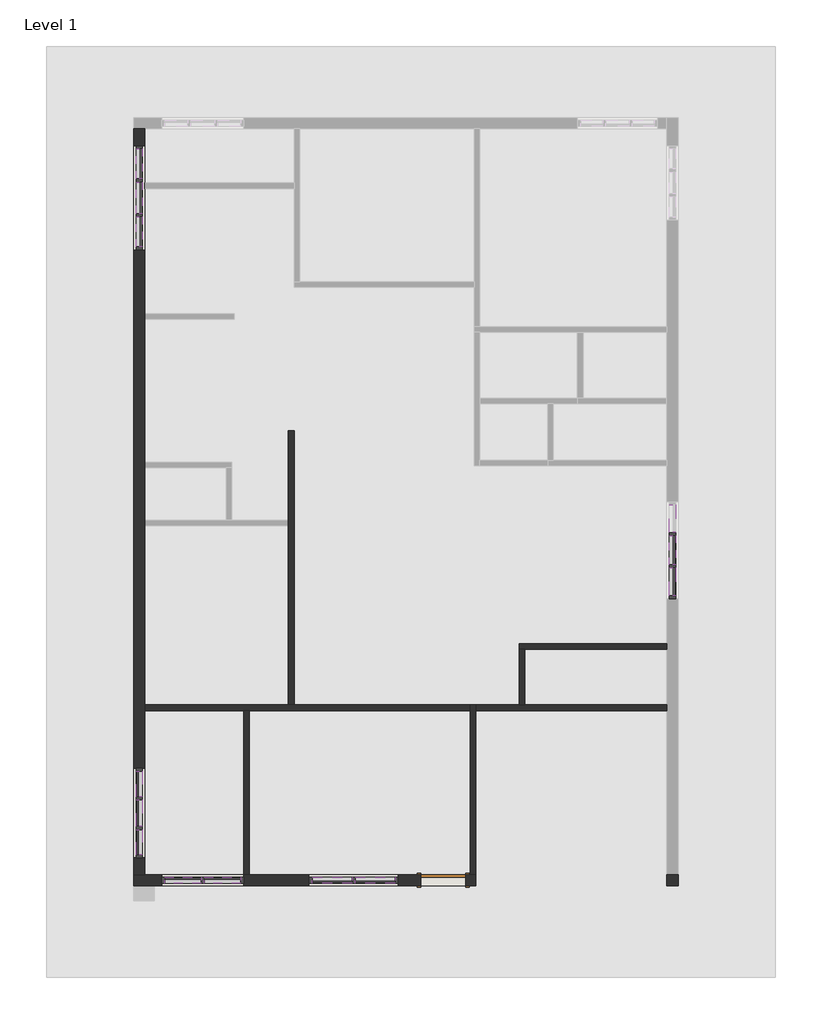
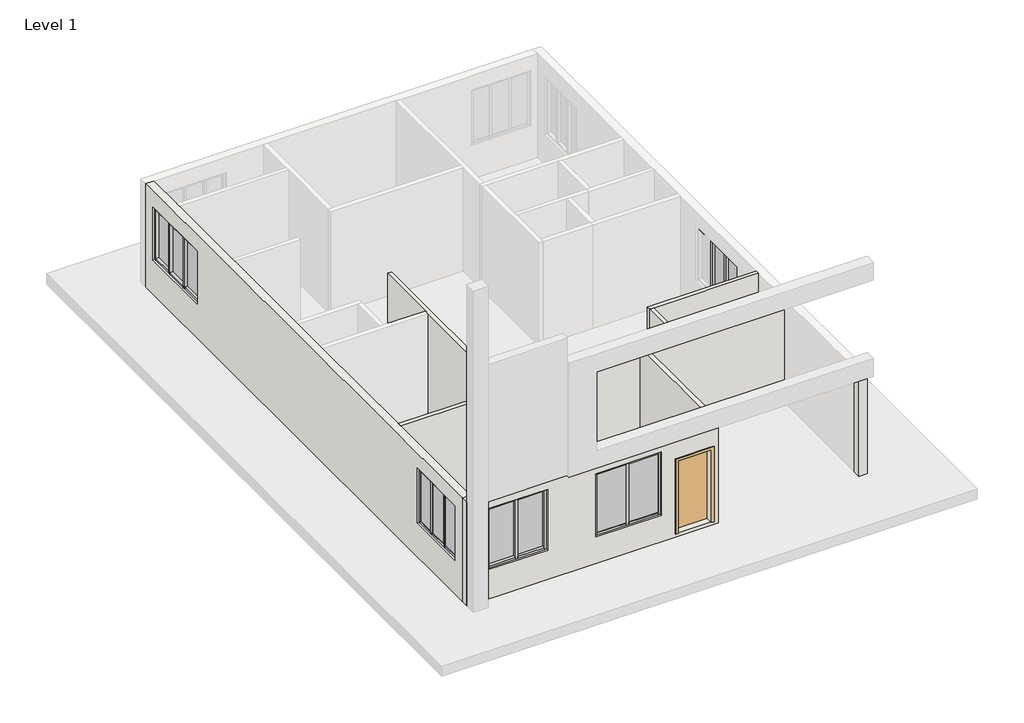
# One storey, part 1 of 2: 42 members, 12 plates, 10 walls, 1 door.
"""IFC4 building model written with IfcOpenShell, lengths in millimetres."""

from ifc_helpers import new_model, si_unit, origin, origin_with_axes, place, context, project, spatial, polyline, outline, extrude, faceted_brep, transform, mapped, element, save
from components import door_0ca8825f, member_6f432376, member_a400357f, member_9c3de6f4, member_520fb4b3, member_5215b92c, member_3f0e0172, member_3a7ae77e, member_6526e201, member_0b7646a3, member_196396ae, member_46a214c3, member_a980948f, member_c17f1be2, member_18118615, member_b3eff8b9, member_3a0a7659, member_3054d540, member_89344730, system_panel_glazed_22e8721b, system_panel_glazed_761c0abc, system_panel_glazed_28bcf516, system_panel_glazed_9d10e14a, system_panel_glazed_438a3505, system_panel_glazed_47776199, system_panel_glazed_6affd56b, system_panel_glazed_c6240b01

model = new_model("IFC4")

# Units and contexts
model_context = context("Model", 3, world=origin())
ifc_project = project(units=[si_unit("LENGTHUNIT", "METRE", prefix="MILLI")], contexts=[model_context])

# Site, building, storey
site = spatial("IfcSite", under=ifc_project)
building = spatial("IfcBuilding", under=site)
storey = spatial("IfcBuildingStorey", under=building, Name="Level 1", Elevation=0.0)

# Door
placement = place(None, origin())
door_shape = door_0ca8825f(model_context)
element("IfcDoor", 1, ObjectType="Single-Flush : 36\" x 84\"", at=placement, inside=storey, context=model_context, shape_type="MappedRepresentation", body=[
    mapped(door_shape, transform((-10676.5767684, -15219.4742702, 101.6), x_axis=(1.0, 0.0, 0.0), y_axis=(0.0, 1.0, 0.0), z_axis=(0.0, 0.0, 1.0))),
])

# Members
member_shape = member_6f432376(model_context)
element("IfcMember", 2, ObjectType="Rectangular Mullion : 2.5\" x 5\" rectangular", at=placement, inside=storey, context=model_context, shape_type="MappedRepresentation", body=[
    mapped(member_shape, transform((-5990.2767684, -8113.8242702, 2606.4568752), x_axis=(0.0, 0.0, 1.0), y_axis=(-1.0, 0.0, 0.0), z_axis=(0.0, -1.0, 0.0))),
])
element("IfcMember", 3, ObjectType="Rectangular Mullion : 2.5\" x 5\" rectangular", at=placement, inside=storey, context=model_context, shape_type="MappedRepresentation", body=[
    mapped(member_shape, transform((-5990.2767684, -9402.8742702, 2606.4568752), x_axis=(0.0, 0.0, 1.0), y_axis=(-1.0, 0.0, 0.0), z_axis=(0.0, -1.0, 0.0))),
])
member_2_shape = member_a400357f(model_context)
element("IfcMember", 4, ObjectType="Rectangular Mullion : 2.5\" x 5\" rectangular", at=placement, inside=storey, context=model_context, shape_type="MappedRepresentation", body=[
    mapped(member_2_shape, transform((-5990.2767684, -8774.2242702, 2606.4568752), x_axis=(0.0, 0.0, 1.0), y_axis=(-1.0, 0.0, 0.0), z_axis=(0.0, -1.0, 0.0))),
])
member_3_shape = member_9c3de6f4(model_context)
element("IfcMember", 5, ObjectType="Rectangular Mullion : 2.5\" x 5\" rectangular", at=placement, inside=storey, context=model_context, shape_type="MappedRepresentation", body=[
    mapped(member_3_shape, transform((-5990.2767684, -8145.5742702, 1004.9988244), x_axis=(0.0, -1.0, 0.0), y_axis=(-1.0, 0.0, 0.0), z_axis=(0.0, 0.0, -1.0))),
])
element("IfcMember", 6, ObjectType="Rectangular Mullion : 2.5\" x 5\" rectangular", at=placement, inside=storey, context=model_context, shape_type="MappedRepresentation", body=[
    mapped(member_3_shape, transform((-5990.2767684, -8805.9742702, 1004.9988244), x_axis=(0.0, -1.0, 0.0), y_axis=(-1.0, 0.0, 0.0), z_axis=(0.0, 0.0, -1.0))),
])
element("IfcMember", 7, ObjectType="Rectangular Mullion : 2.5\" x 5\" rectangular", at=placement, inside=storey, context=model_context, shape_type="MappedRepresentation", body=[
    mapped(member_2_shape, transform((-5990.2767684, -8177.3242702, 1004.9988244), x_axis=(0.0, 0.0, -1.0), y_axis=(-1.0, 0.0, 0.0), z_axis=(0.0, 1.0, 0.0))),
])
element("IfcMember", 8, ObjectType="Rectangular Mullion : 2.5\" x 5\" rectangular", at=placement, inside=storey, context=model_context, shape_type="MappedRepresentation", body=[
    mapped(member_shape, transform((-5990.2767684, -8837.7242702, 1004.9988244), x_axis=(0.0, 0.0, -1.0), y_axis=(-1.0, 0.0, 0.0), z_axis=(0.0, 1.0, 0.0))),
])
member_4_shape = member_520fb4b3(model_context)
element("IfcMember", 9, ObjectType="Rectangular Mullion : 2.5\" x 5\" rectangular", at=placement, inside=storey, context=model_context, shape_type="MappedRepresentation", body=[
    mapped(member_4_shape, transform((-5990.2767684, -9466.3742702, 1004.9988244), x_axis=(0.0, -1.0, 0.0), y_axis=(-1.0, 0.0, 0.0), z_axis=(0.0, 0.0, -1.0))),
])
member_5_shape = member_5215b92c(model_context)
element("IfcMember", 10, ObjectType="Rectangular Mullion : 2.5\" x 5\" rectangular", at=placement, inside=storey, context=model_context, shape_type="MappedRepresentation", body=[
    mapped(member_5_shape, transform((-16886.8767684, -1598.7242702, 2569.033555), x_axis=(0.0, 0.0, 1.0), y_axis=(-1.0, 0.0, 0.0), z_axis=(0.0, -1.0, 0.0))),
])
member_6_shape = member_3f0e0172(model_context)
element("IfcMember", 11, ObjectType="Rectangular Mullion : 2.5\" x 5\" rectangular", at=placement, inside=storey, context=model_context, shape_type="MappedRepresentation", body=[
    mapped(member_6_shape, transform((-16886.8767684, -887.5242702, 2569.033555), x_axis=(0.0, 0.0, 1.0), y_axis=(-1.0, 0.0, 0.0), z_axis=(0.0, -1.0, 0.0))),
])
element("IfcMember", 12, ObjectType="Rectangular Mullion : 2.5\" x 5\" rectangular", at=placement, inside=storey, context=model_context, shape_type="MappedRepresentation", body=[
    mapped(member_6_shape, transform((-16886.8767684, -2278.1742702, 2569.033555), x_axis=(0.0, 0.0, 1.0), y_axis=(-1.0, 0.0, 0.0), z_axis=(0.0, -1.0, 0.0))),
])
member_7_shape = member_3a7ae77e(model_context)
element("IfcMember", 13, ObjectType="Rectangular Mullion : 2.5\" x 5\" rectangular", at=placement, inside=storey, context=model_context, shape_type="MappedRepresentation", body=[
    mapped(member_7_shape, transform((-16886.8767684, -1630.4742702, 1012.5549771), x_axis=(0.0, -1.0, 0.0), y_axis=(-1.0, 0.0, 0.0), z_axis=(0.0, 0.0, -1.0))),
])
element("IfcMember", 14, ObjectType="Rectangular Mullion : 2.5\" x 5\" rectangular", at=placement, inside=storey, context=model_context, shape_type="MappedRepresentation", body=[
    mapped(member_7_shape, transform((-16886.8767684, -919.2742702, 1012.5549771), x_axis=(0.0, -1.0, 0.0), y_axis=(-1.0, 0.0, 0.0), z_axis=(0.0, 0.0, -1.0))),
])
element("IfcMember", 15, ObjectType="Rectangular Mullion : 2.5\" x 5\" rectangular", at=placement, inside=storey, context=model_context, shape_type="MappedRepresentation", body=[
    mapped(member_5_shape, transform((-16886.8767684, -951.0242702, 1012.5549771), x_axis=(0.0, 0.0, -1.0), y_axis=(-1.0, 0.0, 0.0), z_axis=(0.0, 1.0, 0.0))),
])
element("IfcMember", 16, ObjectType="Rectangular Mullion : 2.5\" x 5\" rectangular", at=placement, inside=storey, context=model_context, shape_type="MappedRepresentation", body=[
    mapped(member_6_shape, transform((-16886.8767684, -1662.2242702, 1012.5549771), x_axis=(0.0, 0.0, -1.0), y_axis=(-1.0, 0.0, 0.0), z_axis=(0.0, 1.0, 0.0))),
])
element("IfcMember", 17, ObjectType="Rectangular Mullion : 2.5\" x 5\" rectangular", at=placement, inside=storey, context=model_context, shape_type="MappedRepresentation", body=[
    mapped(member_6_shape, transform((-16886.8767684, -271.5742702, 1012.5549771), x_axis=(0.0, 0.0, -1.0), y_axis=(-1.0, 0.0, 0.0), z_axis=(0.0, 1.0, 0.0))),
])
member_8_shape = member_6526e201(model_context)
element("IfcMember", 18, ObjectType="Rectangular Mullion : 2.5\" x 5\" rectangular", at=placement, inside=storey, context=model_context, shape_type="MappedRepresentation", body=[
    mapped(member_8_shape, transform((-16886.8767684, -2341.6742702, 1012.5549771), x_axis=(0.0, -1.0, 0.0), y_axis=(-1.0, 0.0, 0.0), z_axis=(0.0, 0.0, -1.0))),
])
element("IfcMember", 19, ObjectType="Rectangular Mullion : 2.5\" x 5\" rectangular", at=placement, inside=storey, context=model_context, shape_type="MappedRepresentation", body=[
    mapped(member_8_shape, transform((-16886.8767684, -208.0742702, 2569.033555), x_axis=(0.0, 1.0, 0.0), y_axis=(-1.0, 0.0, 0.0), z_axis=(0.0, 0.0, 1.0))),
])
member_9_shape = member_0b7646a3(model_context)
element("IfcMember", 20, ObjectType="Rectangular Mullion : 2.5\" x 5\" rectangular", at=placement, inside=storey, context=model_context, shape_type="MappedRepresentation", body=[
    mapped(member_9_shape, transform((-16886.8767684, -14184.4242702, 2605.5977524), x_axis=(0.0, 0.0, 1.0), y_axis=(1.0, 0.0, 0.0), z_axis=(0.0, 1.0, 0.0))),
])
element("IfcMember", 21, ObjectType="Rectangular Mullion : 2.5\" x 5\" rectangular", at=placement, inside=storey, context=model_context, shape_type="MappedRepresentation", body=[
    mapped(member_9_shape, transform((-16886.8767684, -12996.9742702, 2605.5977524), x_axis=(0.0, 0.0, 1.0), y_axis=(1.0, 0.0, 0.0), z_axis=(0.0, 1.0, 0.0))),
])
member_10_shape = member_196396ae(model_context)
element("IfcMember", 22, ObjectType="Rectangular Mullion : 2.5\" x 5\" rectangular", at=placement, inside=storey, context=model_context, shape_type="MappedRepresentation", body=[
    mapped(member_10_shape, transform((-16886.8767684, -13543.0742702, 998.5522708), x_axis=(0.0, 1.0, 0.0), y_axis=(1.0, 0.0, 0.0), z_axis=(0.0, 0.0, -1.0))),
])
element("IfcMember", 23, ObjectType="Rectangular Mullion : 2.5\" x 5\" rectangular", at=placement, inside=storey, context=model_context, shape_type="MappedRepresentation", body=[
    mapped(member_10_shape, transform((-16886.8767684, -14152.6742702, 998.5522708), x_axis=(0.0, 1.0, 0.0), y_axis=(1.0, 0.0, 0.0), z_axis=(0.0, 0.0, -1.0))),
])
element("IfcMember", 24, ObjectType="Rectangular Mullion : 2.5\" x 5\" rectangular", at=placement, inside=storey, context=model_context, shape_type="MappedRepresentation", body=[
    mapped(member_9_shape, transform((-16886.8767684, -13511.3242702, 998.5522708), x_axis=(0.0, 0.0, -1.0), y_axis=(1.0, 0.0, 0.0), z_axis=(0.0, -1.0, 0.0))),
])
element("IfcMember", 25, ObjectType="Rectangular Mullion : 2.5\" x 5\" rectangular", at=placement, inside=storey, context=model_context, shape_type="MappedRepresentation", body=[
    mapped(member_9_shape, transform((-16886.8767684, -14698.7742702, 998.5522708), x_axis=(0.0, 0.0, -1.0), y_axis=(1.0, 0.0, 0.0), z_axis=(0.0, -1.0, 0.0))),
])
member_11_shape = member_46a214c3(model_context)
element("IfcMember", 26, ObjectType="Rectangular Mullion : 2.5\" x 5\" rectangular", at=placement, inside=storey, context=model_context, shape_type="MappedRepresentation", body=[
    mapped(member_11_shape, transform((-16886.8767684, -12933.4742702, 998.5522708), x_axis=(0.0, 1.0, 0.0), y_axis=(1.0, 0.0, 0.0), z_axis=(0.0, 0.0, -1.0))),
])
member_12_shape = member_a980948f(model_context)
element("IfcMember", 27, ObjectType="Rectangular Mullion : 2.5\" x 5\" rectangular", at=placement, inside=storey, context=model_context, shape_type="MappedRepresentation", body=[
    mapped(member_12_shape, transform((-16886.8767684, -13574.8242702, 2605.5977524), x_axis=(0.0, 0.0, 1.0), y_axis=(1.0, 0.0, 0.0), z_axis=(0.0, 1.0, 0.0))),
])
element("IfcMember", 28, ObjectType="Rectangular Mullion : 2.5\" x 5\" rectangular", at=placement, inside=storey, context=model_context, shape_type="MappedRepresentation", body=[
    mapped(member_12_shape, transform((-16886.8767684, -14120.9242702, 998.5522708), x_axis=(0.0, 0.0, -1.0), y_axis=(1.0, 0.0, 0.0), z_axis=(0.0, -1.0, 0.0))),
])
element("IfcMember", 29, ObjectType="Rectangular Mullion : 2.5\" x 5\" rectangular", at=placement, inside=storey, context=model_context, shape_type="MappedRepresentation", body=[
    mapped(member_11_shape, transform((-16886.8767684, -14762.2742702, 2605.5977524), x_axis=(0.0, -1.0, 0.0), y_axis=(1.0, 0.0, 0.0), z_axis=(0.0, 0.0, 1.0))),
])
member_13_shape = member_c17f1be2(model_context)
element("IfcMember", 30, ObjectType="Rectangular Mullion : 2.5\" x 5\" rectangular", at=placement, inside=storey, context=model_context, shape_type="MappedRepresentation", body=[
    mapped(member_13_shape, transform((-12473.6267684, -15219.4742702, 2639.1905967), x_axis=(0.0, 0.0, 1.0), y_axis=(0.0, 1.0, 0.0), z_axis=(-1.0, 0.0, 0.0))),
])
element("IfcMember", 31, ObjectType="Rectangular Mullion : 2.5\" x 5\" rectangular", at=placement, inside=storey, context=model_context, shape_type="MappedRepresentation", body=[
    mapped(member_13_shape, transform((-13356.2767684, -15219.4742702, 2639.1905967), x_axis=(0.0, 0.0, 1.0), y_axis=(0.0, 1.0, 0.0), z_axis=(-1.0, 0.0, 0.0))),
])
member_14_shape = member_18118615(model_context)
element("IfcMember", 32, ObjectType="Rectangular Mullion : 2.5\" x 5\" rectangular", at=placement, inside=storey, context=model_context, shape_type="MappedRepresentation", body=[
    mapped(member_14_shape, transform((-12505.3767684, -15219.4742702, 783.5822291), x_axis=(-1.0, 0.0, 0.0), y_axis=(0.0, 1.0, 0.0), z_axis=(0.0, 0.0, -1.0))),
])
element("IfcMember", 33, ObjectType="Rectangular Mullion : 2.5\" x 5\" rectangular", at=placement, inside=storey, context=model_context, shape_type="MappedRepresentation", body=[
    mapped(member_13_shape, transform((-12537.1267684, -15219.4742702, 783.5822291), x_axis=(0.0, 0.0, -1.0), y_axis=(0.0, 1.0, 0.0), z_axis=(1.0, 0.0, 0.0))),
])
element("IfcMember", 34, ObjectType="Rectangular Mullion : 2.5\" x 5\" rectangular", at=placement, inside=storey, context=model_context, shape_type="MappedRepresentation", body=[
    mapped(member_13_shape, transform((-11654.4767684, -15219.4742702, 783.5822291), x_axis=(0.0, 0.0, -1.0), y_axis=(0.0, 1.0, 0.0), z_axis=(1.0, 0.0, 0.0))),
])
member_15_shape = member_b3eff8b9(model_context)
element("IfcMember", 35, ObjectType="Rectangular Mullion : 2.5\" x 5\" rectangular", at=placement, inside=storey, context=model_context, shape_type="MappedRepresentation", body=[
    mapped(member_15_shape, transform((-11590.9767684, -15219.4742702, 2639.1905967), x_axis=(1.0, 0.0, 0.0), y_axis=(0.0, 1.0, 0.0), z_axis=(0.0, 0.0, 1.0))),
])
element("IfcMember", 36, ObjectType="Rectangular Mullion : 2.5\" x 5\" rectangular", at=placement, inside=storey, context=model_context, shape_type="MappedRepresentation", body=[
    mapped(member_15_shape, transform((-13419.7767684, -15219.4742702, 783.5822291), x_axis=(-1.0, 0.0, 0.0), y_axis=(0.0, 1.0, 0.0), z_axis=(0.0, 0.0, -1.0))),
])
member_16_shape = member_3a0a7659(model_context)
element("IfcMember", 37, ObjectType="Rectangular Mullion : 2.5\" x 5\" rectangular", at=placement, inside=storey, context=model_context, shape_type="MappedRepresentation", body=[
    mapped(member_16_shape, transform((-15623.2267684, -15219.4742702, 2655.6153549), x_axis=(0.0, 0.0, 1.0), y_axis=(0.0, -1.0, 0.0), z_axis=(1.0, 0.0, 0.0))),
])
element("IfcMember", 38, ObjectType="Rectangular Mullion : 2.5\" x 5\" rectangular", at=placement, inside=storey, context=model_context, shape_type="MappedRepresentation", body=[
    mapped(member_16_shape, transform((-14816.7767684, -15219.4742702, 2655.6153549), x_axis=(0.0, 0.0, 1.0), y_axis=(0.0, -1.0, 0.0), z_axis=(1.0, 0.0, 0.0))),
])
member_17_shape = member_3054d540(model_context)
element("IfcMember", 39, ObjectType="Rectangular Mullion : 2.5\" x 5\" rectangular", at=placement, inside=storey, context=model_context, shape_type="MappedRepresentation", body=[
    mapped(member_17_shape, transform((-15591.4767684, -15219.4742702, 862.7616395), x_axis=(1.0, 0.0, 0.0), y_axis=(0.0, -1.0, 0.0), z_axis=(0.0, 0.0, -1.0))),
])
element("IfcMember", 40, ObjectType="Rectangular Mullion : 2.5\" x 5\" rectangular", at=placement, inside=storey, context=model_context, shape_type="MappedRepresentation", body=[
    mapped(member_16_shape, transform((-15559.7267684, -15219.4742702, 862.7616395), x_axis=(0.0, 0.0, -1.0), y_axis=(0.0, -1.0, 0.0), z_axis=(-1.0, 0.0, 0.0))),
])
element("IfcMember", 41, ObjectType="Rectangular Mullion : 2.5\" x 5\" rectangular", at=placement, inside=storey, context=model_context, shape_type="MappedRepresentation", body=[
    mapped(member_16_shape, transform((-16366.1767684, -15219.4742702, 862.7616395), x_axis=(0.0, 0.0, -1.0), y_axis=(0.0, -1.0, 0.0), z_axis=(-1.0, 0.0, 0.0))),
])
member_18_shape = member_89344730(model_context)
element("IfcMember", 42, ObjectType="Rectangular Mullion : 2.5\" x 5\" rectangular", at=placement, inside=storey, context=model_context, shape_type="MappedRepresentation", body=[
    mapped(member_18_shape, transform((-14753.2767684, -15219.4742702, 862.7616395), x_axis=(1.0, 0.0, 0.0), y_axis=(0.0, -1.0, 0.0), z_axis=(0.0, 0.0, -1.0))),
])
element("IfcMember", 43, ObjectType="Rectangular Mullion : 2.5\" x 5\" rectangular", at=placement, inside=storey, context=model_context, shape_type="MappedRepresentation", body=[
    mapped(member_18_shape, transform((-16429.6767684, -15219.4742702, 2655.6153549), x_axis=(-1.0, 0.0, 0.0), y_axis=(0.0, -1.0, 0.0), z_axis=(0.0, 0.0, 1.0))),
])

# Plates
system_panel_glazed_shape = system_panel_glazed_22e8721b(model_context)
element("IfcPlate", 44, ObjectType="System Panel : Glazed", at=placement, inside=storey, context=model_context, shape_type="MappedRepresentation", body=[
    mapped(system_panel_glazed_shape, transform((-5990.2767684, -9120.2992702, 1068.4988244), x_axis=(0.0, -1.0, 0.0), y_axis=(1.0, 0.0, 0.0), z_axis=(0.0, 0.0, 1.0))),
])
system_panel_glazed_2_shape = system_panel_glazed_761c0abc(model_context)
element("IfcPlate", 45, ObjectType="System Panel : Glazed", at=placement, inside=storey, context=model_context, shape_type="MappedRepresentation", body=[
    mapped(system_panel_glazed_2_shape, transform((-5990.2767684, -8475.7742702, 1068.4988244), x_axis=(0.0, -1.0, 0.0), y_axis=(1.0, 0.0, 0.0), z_axis=(0.0, 0.0, 1.0))),
])
system_panel_glazed_3_shape = system_panel_glazed_28bcf516(model_context)
element("IfcPlate", 46, ObjectType="System Panel : Glazed", at=placement, inside=storey, context=model_context, shape_type="MappedRepresentation", body=[
    mapped(system_panel_glazed_3_shape, transform((-16886.8767684, -579.5492702, 1076.0549771), x_axis=(0.0, -1.0, 0.0), y_axis=(1.0, 0.0, 0.0), z_axis=(0.0, 0.0, 1.0))),
])
element("IfcPlate", 47, ObjectType="System Panel : Glazed", at=placement, inside=storey, context=model_context, shape_type="MappedRepresentation", body=[
    mapped(system_panel_glazed_3_shape, transform((-16886.8767684, -1970.1992702, 1076.0549771), x_axis=(0.0, -1.0, 0.0), y_axis=(1.0, 0.0, 0.0), z_axis=(0.0, 0.0, 1.0))),
])
system_panel_glazed_4_shape = system_panel_glazed_9d10e14a(model_context)
element("IfcPlate", 48, ObjectType="System Panel : Glazed", at=placement, inside=storey, context=model_context, shape_type="MappedRepresentation", body=[
    mapped(system_panel_glazed_4_shape, transform((-16886.8767684, -1274.8742702, 1076.0549771), x_axis=(0.0, -1.0, 0.0), y_axis=(1.0, 0.0, 0.0), z_axis=(0.0, 0.0, 1.0))),
])
system_panel_glazed_5_shape = system_panel_glazed_438a3505(model_context)
element("IfcPlate", 49, ObjectType="System Panel : Glazed", at=placement, inside=storey, context=model_context, shape_type="MappedRepresentation", body=[
    mapped(system_panel_glazed_5_shape, transform((-16886.8767684, -14441.5992702, 1062.0522708), x_axis=(0.0, 1.0, 0.0), y_axis=(-1.0, 0.0, 0.0), z_axis=(0.0, 0.0, 1.0))),
])
element("IfcPlate", 50, ObjectType="System Panel : Glazed", at=placement, inside=storey, context=model_context, shape_type="MappedRepresentation", body=[
    mapped(system_panel_glazed_5_shape, transform((-16886.8767684, -13254.1492702, 1062.0522708), x_axis=(0.0, 1.0, 0.0), y_axis=(-1.0, 0.0, 0.0), z_axis=(0.0, 0.0, 1.0))),
])
system_panel_glazed_6_shape = system_panel_glazed_47776199(model_context)
element("IfcPlate", 51, ObjectType="System Panel : Glazed", at=placement, inside=storey, context=model_context, shape_type="MappedRepresentation", body=[
    mapped(system_panel_glazed_6_shape, transform((-16886.8767684, -13847.8742702, 1062.0522708), x_axis=(0.0, 1.0, 0.0), y_axis=(-1.0, 0.0, 0.0), z_axis=(0.0, 0.0, 1.0))),
])
system_panel_glazed_7_shape = system_panel_glazed_6affd56b(model_context)
element("IfcPlate", 52, ObjectType="System Panel : Glazed", at=placement, inside=storey, context=model_context, shape_type="MappedRepresentation", body=[
    mapped(system_panel_glazed_7_shape, transform((-12064.0517684, -15219.4742702, 847.0822291), x_axis=(-1.0, 0.0, 0.0), y_axis=(0.0, -1.0, 0.0), z_axis=(0.0, 0.0, 1.0))),
])
element("IfcPlate", 53, ObjectType="System Panel : Glazed", at=placement, inside=storey, context=model_context, shape_type="MappedRepresentation", body=[
    mapped(system_panel_glazed_7_shape, transform((-12946.7017684, -15219.4742702, 847.0822291), x_axis=(-1.0, 0.0, 0.0), y_axis=(0.0, -1.0, 0.0), z_axis=(0.0, 0.0, 1.0))),
])
system_panel_glazed_8_shape = system_panel_glazed_c6240b01(model_context)
element("IfcPlate", 54, ObjectType="System Panel : Glazed", at=placement, inside=storey, context=model_context, shape_type="MappedRepresentation", body=[
    mapped(system_panel_glazed_8_shape, transform((-15994.7017684, -15219.4742702, 926.2616395), x_axis=(1.0, 0.0, 0.0), y_axis=(0.0, 1.0, 0.0), z_axis=(0.0, 0.0, 1.0))),
])
element("IfcPlate", 55, ObjectType="System Panel : Glazed", at=placement, inside=storey, context=model_context, shape_type="MappedRepresentation", body=[
    mapped(system_panel_glazed_8_shape, transform((-15188.2517684, -15219.4742702, 926.2616395), x_axis=(1.0, 0.0, 0.0), y_axis=(0.0, 1.0, 0.0), z_axis=(0.0, 0.0, 1.0))),
])

# Walls
element("IfcWall", 56, ObjectType="4.5\"", at=placement, inside=storey, context=model_context, shape_type="Brep", body=[
    faceted_brep([(-14638.9767684, -15105.1742702, 0.0), (-14638.9767684, -11752.3742702, 0.0), (-14638.9767684, -11752.3742702, 3048.0), (-14638.9767684, -15105.1742702, 3048.0), (-14753.2767684, -15105.1742702, 0.0), (-14753.2767684, -15105.1742702, 862.7616395), (-14753.2767684, -15105.1742702, 2655.6153549), (-14753.2767684, -15105.1742702, 3048.0), (-14753.2767684, -11752.3742702, 3048.0), (-14753.2767684, -11752.3742702, 0.0)], [[[0, 1, 2, 3]], [[4, 5, 6, 7, 8, 9]], [[1, 0, 4, 9]], [[3, 2, 8, 7]], [[0, 3, 7, 6, 5, 4]], [[2, 1, 9, 8]]]),
])
element("IfcWall", 57, ObjectType="4.5\"", at=placement, inside=storey, context=model_context, shape_type="Brep", body=[
    faceted_brep([(-10124.1267684, -11638.0742702, 0.0), (-13724.5767684, -11638.0742702, 0.0), (-13838.8767684, -11638.0742702, 0.0), (-16772.5767684, -11638.0742702, 0.0), (-16772.5767684, -11638.0742702, 3048.0), (-13838.8767684, -11638.0742702, 3048.0), (-13724.5767684, -11638.0742702, 3048.0), (-10124.1267684, -11638.0742702, 3048.0), (-10124.1267684, -11752.3742702, 0.0), (-10124.1267684, -11752.3742702, 3048.0), (-14638.9767684, -11752.3742702, 3048.0), (-14753.2767684, -11752.3742702, 3048.0), (-16772.5767684, -11752.3742702, 3048.0), (-16772.5767684, -11752.3742702, 0.0), (-14753.2767684, -11752.3742702, 0.0), (-14638.9767684, -11752.3742702, 0.0)], [[[0, 1, 2, 3, 4, 5, 6, 7]], [[8, 9, 10, 11, 12, 13, 14, 15]], [[3, 2, 1, 0, 8, 15, 14, 13]], [[7, 6, 5, 4, 12, 11, 10, 9]], [[4, 3, 13, 12]], [[0, 7, 9, 8]]]),
])
element("IfcWall", 58, ObjectType="4.5\"", at=placement, inside=storey, context=model_context, shape_type="Brep", body=[
    faceted_brep([(-10009.8267684, -15105.1742702, 0.0), (-10009.8267684, -11752.3742702, 0.0), (-10009.8267684, -11638.0742702, 0.0), (-10009.8267684, -11638.0742702, 3048.0), (-10009.8267684, -11752.3742702, 3048.0), (-10009.8267684, -15105.1742702, 3048.0), (-10124.1267684, -15105.1742702, 0.0), (-10124.1267684, -15105.1742702, 3048.0), (-10124.1267684, -11752.3742702, 3048.0), (-10124.1267684, -11638.0742702, 3048.0), (-10124.1267684, -11638.0742702, 0.0), (-10124.1267684, -11752.3742702, 0.0)], [[[0, 1, 2, 3, 4, 5]], [[6, 7, 8, 9, 10, 11]], [[2, 1, 0, 6, 11, 10]], [[5, 4, 3, 9, 8, 7]], [[0, 5, 7, 6]], [[3, 2, 10, 9]]]),
])
element("IfcWall", 59, ObjectType="4.5\"", at=placement, inside=storey, context=model_context, shape_type="Brep", body=[
    faceted_brep([(-10009.8267684, -11752.3742702, 0.0), (-6104.5767684, -11752.3742702, 0.0), (-6104.5767684, -11752.3742702, 3048.0), (-10009.8267684, -11752.3742702, 3048.0), (-10009.8267684, -11638.0742702, 0.0), (-10009.8267684, -11638.0742702, 3048.0), (-9127.1767684, -11638.0742702, 3048.0), (-9012.8767684, -11638.0742702, 3048.0), (-6104.5767684, -11638.0742702, 3048.0), (-6104.5767684, -11638.0742702, 0.0), (-9012.8767684, -11638.0742702, 0.0), (-9127.1767684, -11638.0742702, 0.0)], [[[0, 1, 2, 3]], [[4, 5, 6, 7, 8, 9, 10, 11]], [[1, 0, 4, 11, 10, 9]], [[3, 2, 8, 7, 6, 5]], [[0, 3, 5, 4]], [[2, 1, 9, 8]]]),
])
element("IfcWall", 60, ObjectType="4.5\"", at=placement, inside=storey, context=model_context, shape_type="Brep", body=[
    faceted_brep([(-13724.5767684, -11638.0742702, 0.0), (-13724.5767684, -6037.3742702, 0.0), (-13724.5767684, -6037.3742702, 3048.0), (-13724.5767684, -11638.0742702, 3048.0), (-13838.8767684, -11638.0742702, 0.0), (-13838.8767684, -11638.0742702, 3048.0), (-13838.8767684, -7980.4742702, 3048.0), (-13838.8767684, -7866.1742702, 3048.0), (-13838.8767684, -6037.3742702, 3048.0), (-13838.8767684, -6037.3742702, 0.0), (-13838.8767684, -7866.1742702, 0.0), (-13838.8767684, -7980.4742702, 0.0)], [[[0, 1, 2, 3]], [[4, 5, 6, 7, 8, 9, 10, 11]], [[1, 0, 4, 11, 10, 9]], [[2, 1, 9, 8]], [[3, 2, 8, 7, 6, 5]], [[0, 3, 5, 4]]]),
])
element("IfcWall", 61, ObjectType="4.5\"", at=placement, inside=storey, context=model_context, shape_type="Brep", body=[
    faceted_brep([(-6104.5767684, -10387.1242702, 0.0), (-9127.1767684, -10387.1242702, 0.0), (-9127.1767684, -10387.1242702, 3048.0), (-6104.5767684, -10387.1242702, 3048.0), (-6104.5767684, -10501.4242702, 0.0), (-6104.5767684, -10501.4242702, 3048.0), (-9012.8767684, -10501.4242702, 3048.0), (-9127.1767684, -10501.4242702, 3048.0), (-9127.1767684, -10501.4242702, 0.0), (-9012.8767684, -10501.4242702, 0.0)], [[[0, 1, 2, 3]], [[4, 5, 6, 7, 8, 9]], [[1, 0, 4, 9, 8]], [[3, 2, 7, 6, 5]], [[0, 3, 5, 4]], [[2, 1, 8, 7]]]),
])
element("IfcWall", 62, ObjectType="4.5\"", at=placement, inside=storey, context=model_context, shape_type="SweptSolid", body=[
    extrude(outline(polyline([(-9127.1767684, -11638.0742702), (-9127.1767684, -10501.4242702), (-9012.8767684, -10501.4242702), (-9012.8767684, -11638.0742702), (-9127.1767684, -11638.0742702)])), origin_with_axes(), (0.0, 0.0, 1.0), 3048.0),
])
element("IfcWall", 63, ObjectType="9\"", at=placement, inside=storey, context=model_context, shape_type="Brep", body=[
    faceted_brep([(-17001.1767684, -15333.7742702, 0.0), (-10009.8267684, -15333.7742702, 0.0), (-10009.8267684, -15333.7742702, 3048.0), (-17001.1767684, -15333.7742702, 3048.0), (-10219.3767684, -15333.7742702, 101.6), (-11133.7767684, -15333.7742702, 101.6), (-11133.7767684, -15333.7742702, 2235.2), (-10219.3767684, -15333.7742702, 2235.2), (-11590.9767684, -15333.7742702, 2639.1905967), (-11590.9767684, -15333.7742702, 783.5822291), (-13419.7767684, -15333.7742702, 783.5822291), (-13419.7767684, -15333.7742702, 2639.1905967), (-16429.6767684, -15333.7742702, 862.7616395), (-16429.6767684, -15333.7742702, 2655.6153549), (-14753.2767684, -15333.7742702, 2655.6153549), (-14753.2767684, -15333.7742702, 862.7616395), (-10009.8267684, -15105.1742702, 0.0), (-10124.1267684, -15105.1742702, 0.0), (-14638.9767684, -15105.1742702, 0.0), (-14753.2767684, -15105.1742702, 0.0), (-16772.5767684, -15105.1742702, 0.0), (-17001.1767684, -15105.1742702, 0.0), (-17001.1767684, -15105.1742702, 3048.0), (-16772.5767684, -15105.1742702, 3048.0), (-14753.2767684, -15105.1742702, 3048.0), (-14638.9767684, -15105.1742702, 3048.0), (-10124.1267684, -15105.1742702, 3048.0), (-10009.8267684, -15105.1742702, 3048.0), (-11133.7767684, -15105.1742702, 101.6), (-10219.3767684, -15105.1742702, 101.6), (-10219.3767684, -15105.1742702, 2235.2), (-11133.7767684, -15105.1742702, 2235.2), (-11590.9767684, -15105.1742702, 783.5822291), (-11590.9767684, -15105.1742702, 2639.1905967), (-13419.7767684, -15105.1742702, 2639.1905967), (-13419.7767684, -15105.1742702, 783.5822291), (-16429.6767684, -15105.1742702, 2655.6153549), (-16429.6767684, -15105.1742702, 862.7616395), (-14753.2767684, -15105.1742702, 862.7616395), (-14753.2767684, -15105.1742702, 2655.6153549)], [[[0, 1, 2, 3], [4, 5, 6, 7], [8, 9, 10, 11], [12, 13, 14, 15]], [[16, 17, 18, 19, 20, 21, 22, 23, 24, 25, 26, 27], [28, 29, 30, 31], [32, 33, 34, 35], [36, 37, 38, 39]], [[1, 0, 21, 20, 19, 18, 17, 16]], [[2, 1, 16, 27]], [[3, 2, 27, 26, 25, 24, 23, 22]], [[0, 3, 22, 21]], [[29, 28, 5, 4]], [[30, 29, 4, 7]], [[31, 30, 7, 6]], [[28, 31, 6, 5]], [[32, 9, 8, 33]], [[33, 8, 11, 34]], [[34, 11, 10, 35]], [[9, 32, 35, 10]], [[36, 13, 12, 37]], [[13, 36, 39, 14]], [[14, 39, 38, 15]], [[37, 12, 15, 38]]]),
])
element("IfcWall", 64, ObjectType="9\"", at=placement, inside=storey, context=model_context, shape_type="Brep", body=[
    faceted_brep([(-17001.1767684, 134.8257298, 0.0), (-17001.1767684, -15105.1742702, 0.0), (-17001.1767684, -15105.1742702, 3048.0), (-17001.1767684, 134.8257298, 3048.0), (-17001.1767684, -14762.2742702, 2605.5977524), (-17001.1767684, -14762.2742702, 998.5522708), (-17001.1767684, -12933.4742702, 998.5522708), (-17001.1767684, -12933.4742702, 2605.5977524), (-17001.1767684, -208.0742702, 1012.5549771), (-17001.1767684, -208.0742702, 2569.033555), (-17001.1767684, -2341.6742702, 2569.033555), (-17001.1767684, -2341.6742702, 1012.5549771), (-16772.5767684, -15105.1742702, 0.0), (-16772.5767684, -11752.3742702, 0.0), (-16772.5767684, -11638.0742702, 0.0), (-16772.5767684, -7980.4742702, 0.0), (-16772.5767684, -7866.1742702, 0.0), (-16772.5767684, -6793.0242702, 0.0), (-16772.5767684, -6678.7242702, 0.0), (-16772.5767684, -3757.7242702, 0.0), (-16772.5767684, -3643.4242702, 0.0), (-16772.5767684, -1084.3742702, 0.0), (-16772.5767684, -970.0742702, 0.0), (-16772.5767684, 134.8257298, 0.0), (-16772.5767684, 134.8257298, 3048.0), (-16772.5767684, -970.0742702, 3048.0), (-16772.5767684, -1084.3742702, 3048.0), (-16772.5767684, -3643.4242702, 3048.0), (-16772.5767684, -3757.7242702, 3048.0), (-16772.5767684, -6678.7242702, 3048.0), (-16772.5767684, -6793.0242702, 3048.0), (-16772.5767684, -7866.1742702, 3048.0), (-16772.5767684, -7980.4742702, 3048.0), (-16772.5767684, -11638.0742702, 3048.0), (-16772.5767684, -11752.3742702, 3048.0), (-16772.5767684, -15105.1742702, 3048.0), (-16772.5767684, -14762.2742702, 998.5522708), (-16772.5767684, -14762.2742702, 2605.5977524), (-16772.5767684, -12933.4742702, 2605.5977524), (-16772.5767684, -12933.4742702, 998.5522708), (-16772.5767684, -208.0742702, 2569.033555), (-16772.5767684, -208.0742702, 1012.5549771), (-16772.5767684, -2341.6742702, 1012.5549771), (-16772.5767684, -2341.6742702, 2569.033555)], [[[0, 1, 2, 3], [4, 5, 6, 7], [8, 9, 10, 11]], [[12, 13, 14, 15, 16, 17, 18, 19, 20, 21, 22, 23, 24, 25, 26, 27, 28, 29, 30, 31, 32, 33, 34, 35], [36, 37, 38, 39], [40, 41, 42, 43]], [[1, 0, 23, 22, 21, 20, 19, 18, 17, 16, 15, 14, 13, 12]], [[3, 2, 35, 34, 33, 32, 31, 30, 29, 28, 27, 26, 25, 24]], [[0, 3, 24, 23]], [[2, 1, 12, 35]], [[36, 5, 4, 37]], [[37, 4, 7, 38]], [[6, 39, 38, 7]], [[5, 36, 39, 6]], [[8, 41, 40, 9]], [[9, 40, 43, 10]], [[10, 43, 42, 11]], [[41, 8, 11, 42]]]),
])
element("IfcWall", 65, ObjectType="9\"", at=placement, inside=storey, context=model_context, shape_type="SweptSolid", body=[
    extrude(outline(polyline([(-5875.9767684, -15333.7742702), (-6104.5767684, -15333.7742702), (-6104.5767684, -15105.1742702), (-5875.9767684, -15105.1742702), (-5875.9767684, -15333.7742702)])), origin_with_axes(), (0.0, 0.0, 1.0), 3048.0),
])

save(model, "model.ifc")

# Revit data of these elements
# Type "Single-Flush : 36\" x 84\""
#   Type Mark = "1"
#   Construction Type Id = "MDOOR"
#   Assembly Code = "C1020"
#   Analytic Construction = "Metal"
#   Thickness = 0' - 2"
#   Heat Transfer Coefficient (U) = 0.651978 BTU/(h·ft²·°F)
#   Height = 7' - 0"
#   Trim Projection Ext = 0' - 1"
#   Trim Projection Int = 0' - 1"
#   Trim Width = 0' - 3"
#   Width = 3' - 0"
#   Define Thermal Properties by = 1
#   Define Thermal Properties by = 1
#   Door Material = Door - Panel
#   Frame Material = Door - Frame
#   Visual Light Transmittance = 0
#   Solar Heat Gain Coefficient = 0
#   Function = (empty or 0)
#   Wall Closure = (empty or 0)
# Type "Rectangular Mullion : 2.5\" x 5\" rectangular"
#   built-in parameter 1007304 = 0.416667 (stored number, unit not read)
#   built-in parameter 1007301 = 0.104167 (stored number, unit not read)
#   built-in parameter 1007300 = 0.104167 (stored number, unit not read)
# Type "System Panel : Glazed"
#   Construction Type Id = "GSP4R"
#   Analytic Construction = "1/8 in Pilkington single glazing"
#   Visual Light Transmittance = 0.9
#   Solar Heat Gain Coefficient = 0.86
#   Heat Transfer Coefficient (U) = 1.18115 BTU/(h·ft²·°F)
#   Define Thermal Properties by = 1
# Type "4.5\""
#   Assembly Code = "B2010"
#   Layers, outside or top first: 0' - 4 1/2" no material (function 1)
# Type "9\""
#   Assembly Code = "B2010"
#   Layers, outside or top first: 0' - 9" no material (function 1)
# Element 1 (IfcDoor, "Single-Flush : 36\" x 84\"")
#   Phase Created = New Construction
#   Materials on its faces: "Door - Frame", "Door - Panel"
# Elements 2, 3, 4, 5, 6, 7, 8, 9, 10, 11, 12, 13, 14, 15, 16, 17, 18, 19, 20, 21, 22, 23, 24, 25, 26, 27, 28, 29, 30, 31, 32, 33, 34, 35, 36, 37, 38, 39, 40, 41, 42, 43 (IfcMember, "Rectangular Mullion : 2.5\" x 5\" rectangular")
#   Phase Created = New Construction
#   Materials on its faces: "Aluminum"
# Elements 44, 45, 46, 47, 48, 49, 50, 51, 52, 53, 54, 55 (IfcPlate, "System Panel : Glazed")
#   Phase Created = New Construction
#   Materials on its faces: "Glass"
# Elements 56, 57, 58, 59, 60, 61, 62 (IfcWall, "4.5\"")
#   Top Offset = 0' - 0"
#   Base Offset = 0' - 0"
#   Unconnected Height = 10' - 0"
#   wall height = 10' - 0"
#   Phase Created = New Construction
#   Base Constraint = Level 1
#   Materials on its faces: "Default Wall"
# Elements 63, 64, 65 (IfcWall, "9\"")
#   Top Offset = 0' - 0"
#   Base Offset = 0' - 0"
#   Unconnected Height = 10' - 0"
#   wall height = 10' - 0"
#   Phase Created = New Construction
#   Base Constraint = Level 1
#   Materials on its faces: "Default Wall"
# Materials
#   "Door - Panel": class "Wood", colour RGB 210 159 95, transparency 0, Cost = 0
#   "Door - Frame": colour RGB 118 70 51, transparency 0, Cost = 0
#   "Aluminum": class "Metal", colour RGB 247 247 247, transparency 0, Description = "Aluminum 6061", Cost = 0
#   "Glass": class "Glass", colour RGB 0 128 192, transparency 0.75, Description = "Soda Lime Glass", Cost = 0
#   "Default Wall": colour RGB 128 128 128, transparency 0, Cost = 0
